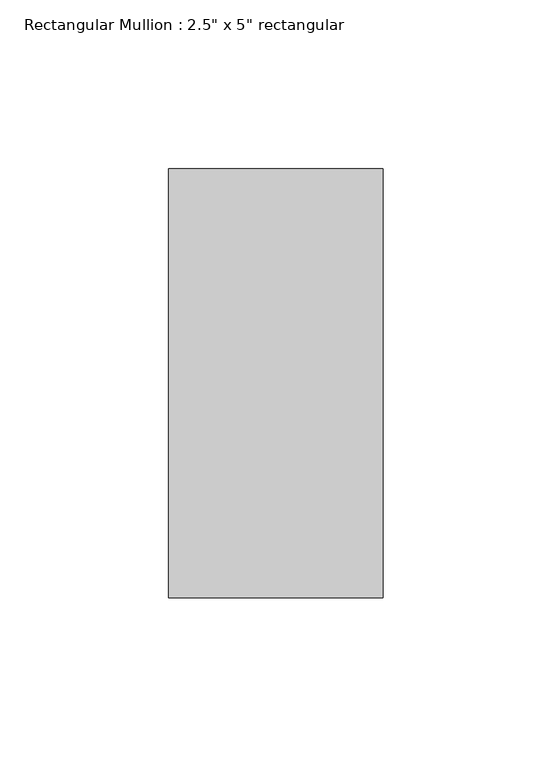
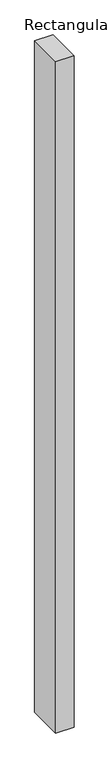
"""IFC4 building model written with IfcOpenShell, lengths in millimetres: member geometry."""

from ifc_helpers import new_model, si_unit, frame, origin, place, context, project, spatial, polyline, outline, extrude, source, transform, mapped, element, save


def member_d4df521d(model_context):
    return source(origin(), model_context, "Body", "SweptSolid", [
        extrude(outline(polyline([(31.75, 63.5), (31.75, -63.5), (-31.75, -63.5), (-31.75, 63.5), (31.75, 63.5)])), frame((0.0, 0.0, -2468.3449309), z_axis=(0.0, 0.0, 1.0), x_axis=(1.0, 0.0, 0.0)), (0.0, 0.0, 1.0), 2468.3449309),
    ])


if __name__ == "__main__":
    model = new_model("IFC4")
    model_context = context("Model", 3, world=origin())
    ifc_project = project(units=[si_unit("LENGTHUNIT", "METRE", prefix="MILLI")], contexts=[model_context])
    site = spatial("IfcSite", under=ifc_project)
    building = spatial("IfcBuilding", under=site)
    placement = place(None, origin())
    member_shape = member_d4df521d(model_context)
    element("IfcMember", 1, ObjectType="Rectangular Mullion : 2.5\" x 5\" rectangular", at=placement, inside=building, context=model_context, shape_type="MappedRepresentation", body=[
        mapped(member_shape, transform((0.0, 0.0, 0.0), x_axis=(1.0, 0.0, 0.0), y_axis=(0.0, 1.0, 0.0), z_axis=(0.0, 0.0, 1.0))),
    ])
    save(model, "model.ifc")

# Revit data of these elements
# Type "Rectangular Mullion : 2.5\" x 5\" rectangular"
#   built-in parameter 1007304 = 0.416667 (stored number, unit not read)
#   built-in parameter 1007301 = 0.104167 (stored number, unit not read)
#   built-in parameter 1007300 = 0.104167 (stored number, unit not read)
# Element 1 (IfcMember, "Rectangular Mullion : 2.5\" x 5\" rectangular")
#   Materials on its faces: "Aluminum"
# Materials
#   "Aluminum": class "Metal", colour RGB 247 247 247, transparency 0, Description = "Aluminum 6061", Cost = 0
